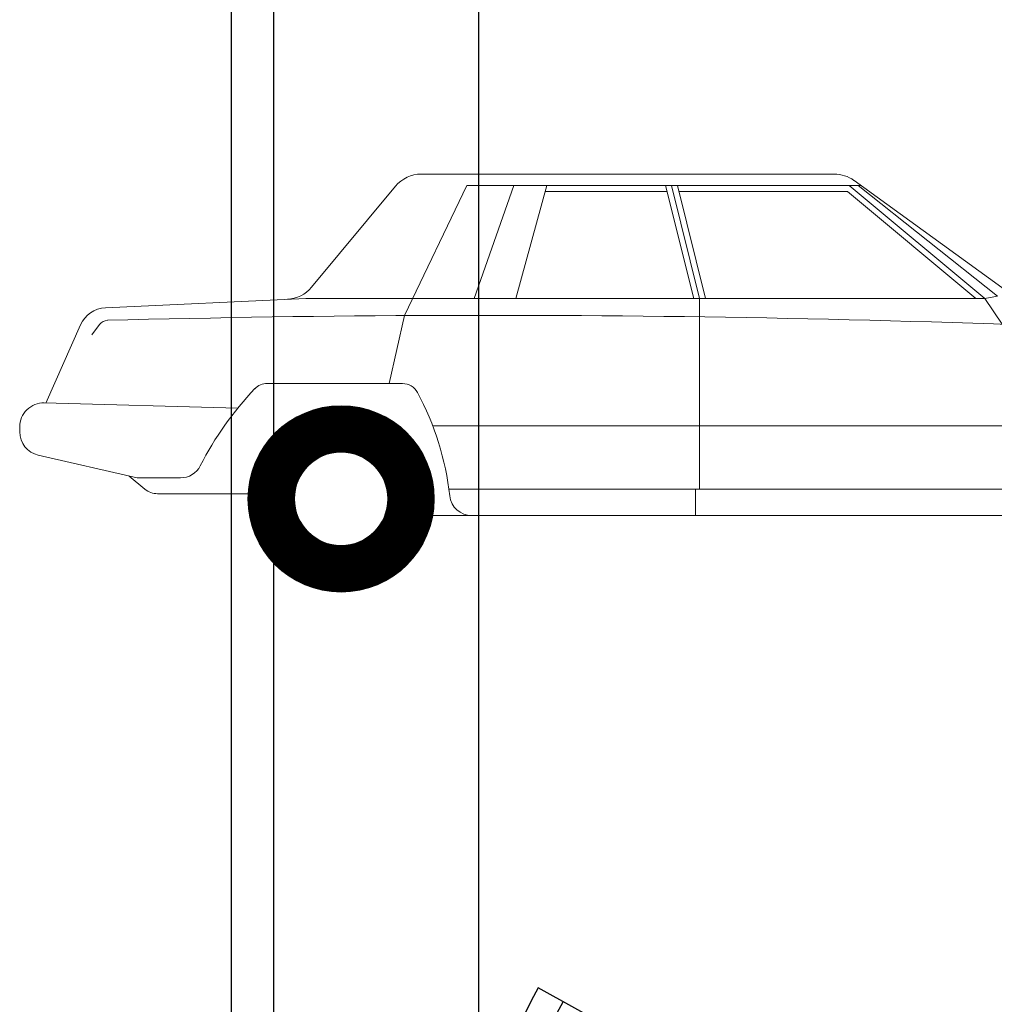
# Model space of a CAD drawing. Units: inches. Extents: x 371 to 1095, y -45 to 1219.
# Tile 5 of 18: x 837 to 952, y 188 to 304. Entities that reach past the tile are written whole.
import ezdxf

# ---------------------------------------------------------------- set-up
doc = ezdxf.new("R2010")
doc.units = ezdxf.units.IN
doc.header["$MEASUREMENT"] = 0
for name, color, linetype, lineweight in [('A-ANNO-DIMS', 2, 'Continuous', 18), ('A-FLOR-STRS', 7, 'Continuous', 25), ('C-SITE-VEHC', 8, 'Continuous', 18)]:
    doc.layers.add(name, color=color, linetype=linetype, lineweight=lineweight)
doc.styles.get("Standard").update_dxf_attribs({"font": 'arial.ttf'})
doc.dimstyles.get("Standard").update_dxf_attribs({"dimtxt": 1, "dimasz": 1, "dimexe": 0.18, "dimexo": 0.0625, "dimgap": 0.09, "dimtad": 0, "dimtih": 1, "dimtoh": 1, "dimdec": 0, "dimzin": 0, "dimdsep": 46, "dimlunit": 3, "dimtxsty": 'Standard', "dimcen": 0.09, "dimadec": 0, "dimazin": 0, "dimtfac": 1, "dimtdec": 0, "dimtofl": 0, "dimtmove": 0, "dimatfit": 3, "dimfxl": 1, "dimtolj": 1, "dimtzin": 0, "dimarcsym": 0})

# ---------------------------------------------------------------- blocks, each defined once
blk = doc.blocks.new('Staircase - Spiral')
blk.add_line((0, 4.5), (0, 30))
for radius in [30, 28.5]:
    blk.add_arc((0, 0), radius, 90, 0)
blk = doc.blocks.new('Car - sedan  side')
for p, q in [((-77.81, 49.34), (-126.58, 49.34)), ((-139.53, 35.99), (-129.64, 47.91)), ((-128.57, 32.64), (-121.22, 48.02)), ((-74.7, 48.02), (-121.22, 48.02)), ((-120.32, 34.67), (-115.67, 48.02)), ((-115.4, 34.67), (-111.74, 48.02)), ((-94.41, 34.67), (-97.73, 48.02)), ((-93.72, 34.67), (-97.04, 48.02)), ((-93.03, 34.67), (-96.34, 48.02)), ((-60.02, 34.65), (-76.07, 48.02)), ((-56.87, 35.13), (-75.48, 48.59)), ((-58.54, 34.93), (-74.99, 48.02)), ((-97.55, 47.3), (-111.94, 47.3)), ((-76.26, 47.3), (-96.16, 47.3)), ((-61.08, 34.66), (-76.26, 47.3)), ((-60.02, 34.65), (-58.54, 34.93)), ((-140.23, 34.67), (-163.88, 33.56)), ((-62.28, 34.67), (-140.23, 34.67)), ((-93.72, 19.62), (-93.72, 34.67)), ((-62.28, 34.67), (-60.02, 34.65)), ((-57.97, 31.61), (-60.02, 34.65)), ((-130.39, 24.63), (-128.57, 32.64)), ((-170.93, 22.32), (-166.81, 31.56)), ((-164.57, 31.6), (-165.48, 30.35)), ((-128.78, 24.63), (-144.79, 24.63)), ((-148.26, 21.7), (-171.11, 22.33)), ((-174, 19.51), (-174, 18.91)), ((-47.2, 19.62), (-125.23, 19.62)), ((-93.72, 12.14), (-93.72, 19.62)), ((-160.12, 13.48), (-171.81, 16.16)), ((-159.22, 12.14), (-161.08, 13.7)), ((-155.01, 13.48), (-160.12, 13.48)), ((-50.67, 12.14), (-123.32, 12.14)), ((-94.21, 9.03), (-94.21, 12.14)), ((-147.03, 11.6), (-157.73, 11.6)), ((-120.62, 9.03), (-125.23, 9.03)), ((-45.76, 9.03), (-120.62, 9.03))]:
    blk.add_line(p, q)
at = {"const_width": 5.49}
blk.add_lwpolyline([(-127.8, 11, -1), (-144.3, 11, -1)], format="xyb", close=True, dxfattribs=at)
for radius in [11, 5.51]:
    blk.add_circle((-136.05, 11), radius)
for centre, radius, start, end in [((-126.58, 45.38), 3.97, 90, 140.3029), ((-77.81, 45.38), 3.97, 54.135, 90), ((-142.58, 38.53), 3.97, 272.6827, 320.3029), ((-163.72, 30.18), 3.38, 92.6827, 155.9736), ((-118.51, -1702.12), 1734.79, 86.34698, 91.49105), ((-163.62, 30.91), 1.17, 91.491, 143.9553), ((-144.79, 22.64), 1.98, 90, 136.3964), ((-128.78, 22.64), 1.98, 28.1371, 90), ((-118.09, -2.78), 38.85, 136.3964, 152.9097), ((-157.14, 7.48), 34.14, 6.5135, 28.1371), ((-171.18, 19.51), 2.82, 88.4193, 180), ((-171.18, 18.91), 2.82, 180, 257.0905), ((-155.01, 16.1), 2.62, 270, 332.9097), ((-157.73, 13.93), 2.32, 230.1291, 270), ((-120.62, 11.65), 2.62, 186.5135, 270)]:
    blk.add_arc(centre, radius, start, end)
blk = doc.blocks.new('*D60')
at = {"layer": 'A-ANNO-DIMS', "color": 0, "lineweight": -2, "transparency": 16777216}
for p, q in [((866.81, 441.96), (866.81, -43.83)), ((891.01, 441.96), (891.01, -43.83)), ((867.81, -43.65), (877.48, -43.65)), ((890.01, -43.65), (880.33, -43.65))]:
    blk.add_line(p, q, dxfattribs=at)
at = {"layer": 'A-ANNO-DIMS', "color": 0, "transparency": 16777216}
for points in [[(867.81, -43.48), (867.81, -43.82), (866.81, -43.65)], [(890.01, -43.48), (890.01, -43.82), (891.01, -43.65)]]:
    blk.add_solid(points, dxfattribs=at)
at = {"layer": 'Defpoints', "color": 0, "transparency": 16777216}
for p in [(866.81, 442.03), (891.01, 442.03), (891.01, -43.65)]:
    blk.add_point(p, dxfattribs=at)
at = {"layer": 'A-ANNO-DIMS', "color": 0, "transparency": 16777216, "insert": (878.91, -43.65), "char_height": 1, "attachment_point": 5}
blk.add_mtext('\\A1;2\'-0"', dxfattribs=at)
blk = doc.blocks.new('*D61')
at = {"layer": 'A-ANNO-DIMS', "color": 0, "lineweight": -2, "transparency": 16777216}
for p, q in [((861.81, 450.96), (861.81, -43.83)), ((866.81, 450.96), (866.81, -43.83)), ((860.81, -43.65), (859.81, -43.65)), ((867.81, -43.65), (868.81, -43.65))]:
    blk.add_line(p, q, dxfattribs=at)
at = {"layer": 'A-ANNO-DIMS', "color": 0, "transparency": 16777216}
for points in [[(860.81, -43.48), (860.81, -43.82), (861.81, -43.65)], [(867.81, -43.48), (867.81, -43.82), (866.81, -43.65)]]:
    blk.add_solid(points, dxfattribs=at)
at = {"layer": 'Defpoints', "color": 0, "transparency": 16777216}
for p in [(861.81, 451.03), (866.81, 451.03), (866.81, -43.65)]:
    blk.add_point(p, dxfattribs=at)
at = {"layer": 'A-ANNO-DIMS', "color": 0, "transparency": 16777216, "insert": (864.31, -43.65), "char_height": 1, "attachment_point": 5}
blk.add_mtext('\\A1;0\'-5"', dxfattribs=at)

msp = doc.modelspace()

# ---------------------------------------------------------------- block references
at = {"layer": 'A-FLOR-STRS', "xscale": 2.233824712970382, "yscale": 2.233824712970382, "zscale": 2.233824712970382, "rotation": 61.2124779579666}
msp.add_blockref('Staircase - Spiral', (956.78, 157.87), dxfattribs=at)
at = {"layer": 'C-SITE-VEHC'}
msp.add_blockref('Car - sedan  side', (1010.83, 236.89), dxfattribs=at)

# ---------------------------------------------------------------- dimensions: what is measured, and where the dimension line sits
at = {"layer": 'A-ANNO-DIMS'}
for base, p1, p2, picture, middle in [((866.81, -43.65), (861.81, 451.03), (866.81, 451.03), '*D61', (864.31, -43.65)), ((891.01, -43.65), (866.81, 442.03), (891.01, 442.03), '*D60', (878.91, -43.65))]:
    dim = msp.add_linear_dim(base=base, p1=p1, p2=p2, dimstyle='Standard', override={"dimdec": 1, "dimlfac": 1, "dimrnd": 0, "dimzin": 1, "dimdsep": 46, "dimlunit": 4, "dimfrac": 2}, dxfattribs=at)
    dim.commit()
    dim.dimension.update_dxf_attribs({"geometry": picture, "text_midpoint": middle})

doc.saveas('drawing.dxf')
